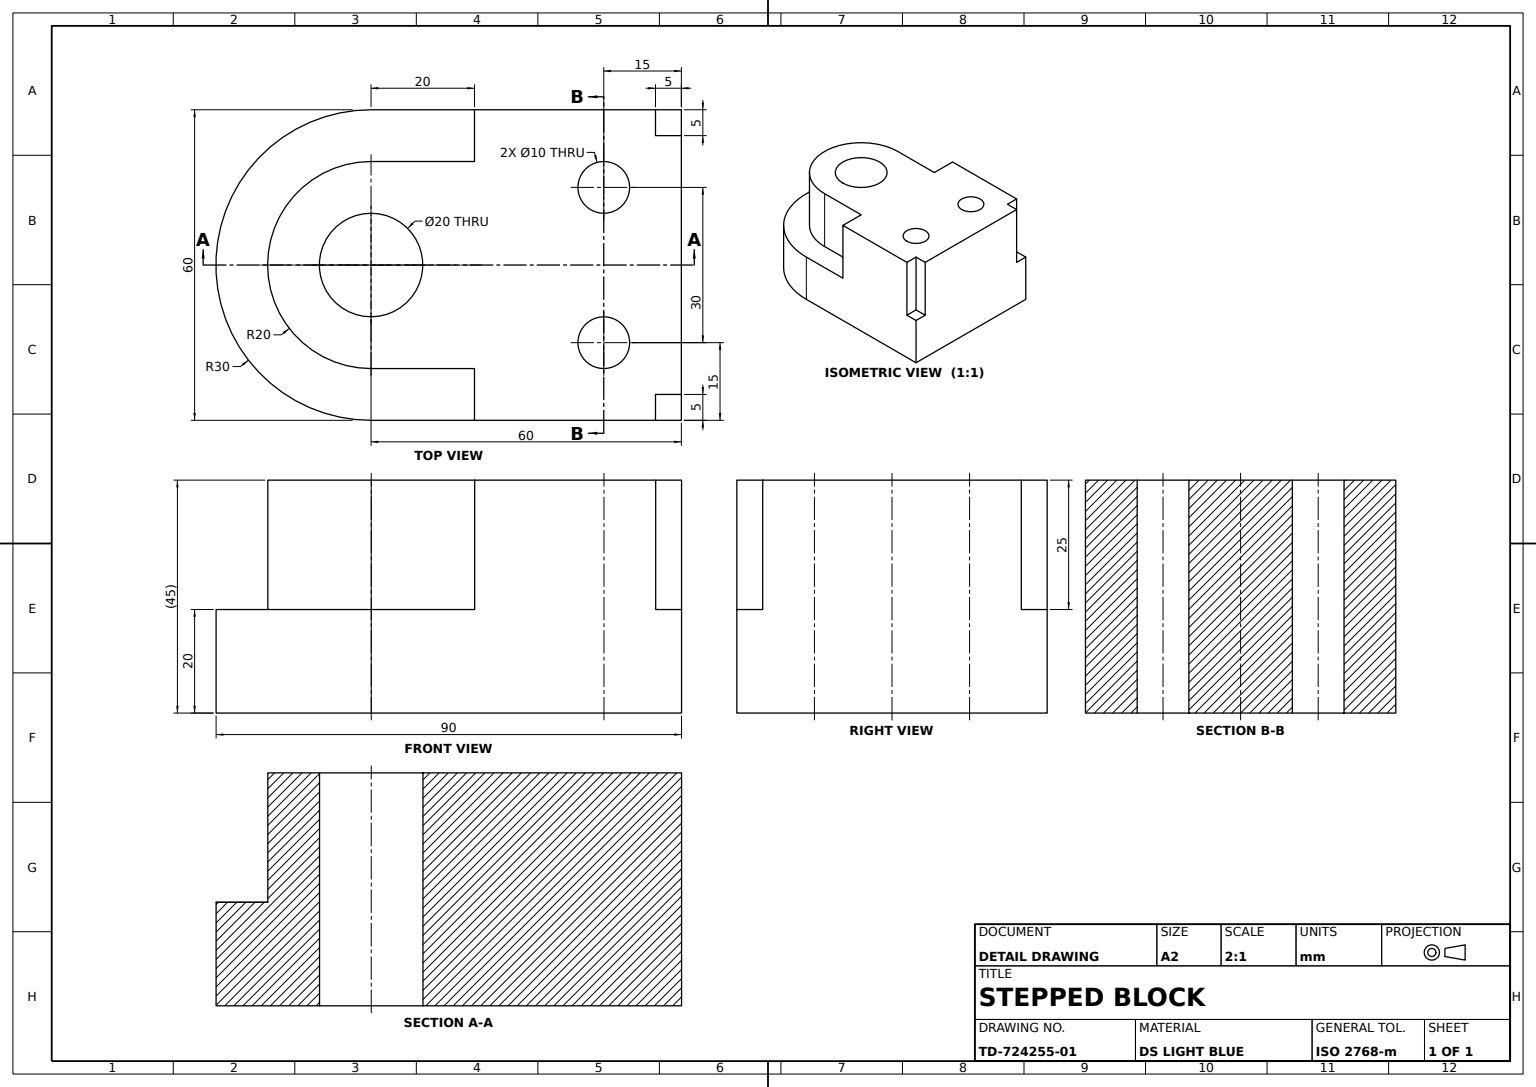
CATIA V5 part; units mm, degrees
sketch "Sketch1" plane through (0, 0, 0) normal (0, 0, 1) x (0, 1, 0)
  line L0 (30, 30) -> (30, -30)
  line L1 (30, -30) -> (-30, -30)
  line L2 (-30, -30) -> (-30, 30) construction
  line L3 (-30, 30) -> (30, 30)
  arc A0 (-30, -30) -> (-30, 30) centre (-30, 0) cw
  point P0 (-60, 0)
  dimension "length L0" = 60
  dimension "length L3" = 60
  constraint vertical L0 y-axis
  constraint vertical L2 y-axis
  constraint horizontal L1 x-axis
  constraint horizontal L3 x-axis
  constraint equidistance L0 L2 origin
  constraint equidistance L1 L3 origin
  constraint coincidence A0 P0
  constraint coincidence P0 x-axis
  constraint tangency L3 A0
  constraint tangency L1 A0
extrude "Pad1" add sketch "Sketch1" along normal blind 20
sketch "Sketch2" plane through (0, 0, 20) normal (0, 0, 1) x (1, 0, 0)
  line L0 (30, -30) -> (30, 30) construction
  line L1 (30, -10) -> (30, 25)
  point P0 (30, -30)
  line L2 (30, 30) -> (-30, 30) construction
  line L3 (25, 30) -> (-25, 30)
  line L4 (-30, 25) -> (-25, 25)
  line L5 (-25, 25) -> (-25, 30)
  point P1 (-25, 30)
  point P2 (25, 30)
  line L6 (30, 25) -> (25, 25)
  line L7 (25, 25) -> (25, 30)
  point P3 (30, 25)
  point P4 (0, -50)
  line L8 (-30, 30) -> (-30, -30) construction
  line L9 (-30, 25) -> (-30, -10)
  point P5 (30, -10)
  line L10 (30, -10) -> (20, -10)
  point P6 (20, -10)
  point P7 (-20, -10)
  line L11 (-20, -10) -> (-30, -10)
  point P8 (-30, -10)
  line L12 (20, -10) -> (20, -30)
  arc A0 (20, -30) -> (-20, -30) centre (0, -30) cw
  line L13 (-20, -30) -> (-20, -10)
  arc A1 (-30, -30) -> (30, -30) centre (0, -30) ccw construction
  dimension "length L6" = 5
  dimension "length L7" = 5
  dimension "length L5" = 5
  dimension "length L4" = 5
  dimension "distance P0 L10" = 20
  dimension "radius A0" = 20
  constraint horizontal L4 x-axis
  constraint horizontal L6 x-axis
  constraint horizontal L10 x-axis
  constraint horizontal L11 x-axis
  constraint vertical L5 y-axis
  constraint vertical L7 y-axis
  constraint vertical L12 y-axis
  constraint coincidence P1 L2
  constraint coincidence P2 L2
  constraint coincidence P3 L0
  constraint coincidence P5 L0
  constraint coincidence P8 L8
  constraint symmetry P6 P7 y-axis
  constraint tangency A0 L12
  constraint tangency L13 A0
  constraint concentricity A0 A1
extrude "Pad2" add sketch "Sketch2" along normal blind 25
sketch "Sketch3" plane through (0, 0, 45) normal (0, 0, 1) x (0, 1, 0)
  circle A0 centre (-30, 0) radius 10
  point P0 (-30, 0)
  circle A1 centre (15, 15) radius 5
  point P1 (15, 15)
  circle A2 centre (15, -15) radius 5
  point P2 (15, -15)
  arc A3 (-30, 19.9664) -> (-30, -19.9664) centre (-28.8406, 0) ccw construction
  line L0 (30, 23.8406) -> (30, -23.8406) construction
  arc A4 (-30, 20) -> (-30, -20) centre (-30, 0) ccw construction
  dimension "radius A0" = 10
  dimension "radius A2" = 5
  dimension "radius A1" = 5
  dimension "distance P2 P1" = 30
  dimension "distance P2 L0" = 15
  constraint coincidence P0 x-axis
  constraint symmetry P1 P2 x-axis
  constraint concentricity A0 A4
extrude "Pocket1" cut sketch "Sketch3" against normal through all
properties material "DS Light Blue"
